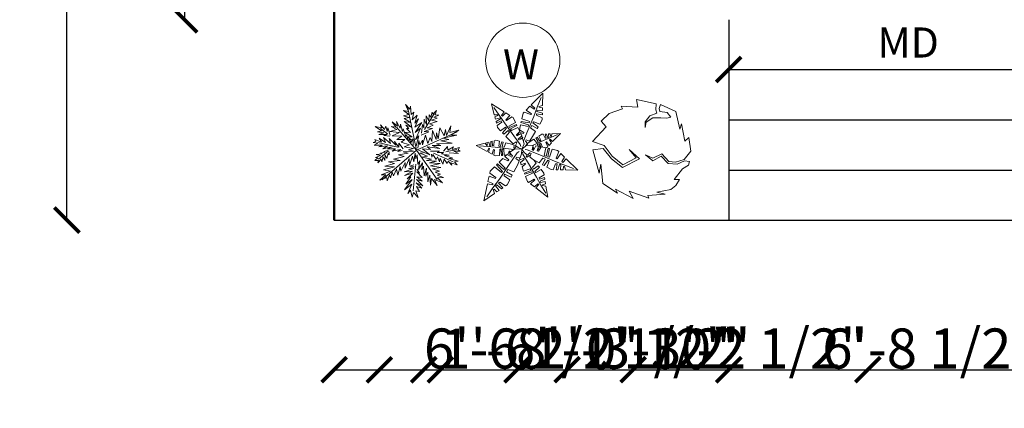
# Model space of a CAD drawing. Units: inches. Extents: x 2169 to 2662, y 1518 to 2151.
# Tile 1 of 6: x 2201 to 2398, y 1518 to 1596. Entities that reach past the tile are written whole.
import ezdxf

# ---------------------------------------------------------------- set-up
doc = ezdxf.new("R2010")
doc.units = ezdxf.units.IN
for name, color, linetype, lineweight in [('A-ANNO-DIMS', 2, 'Continuous', 18), ('A-ANNO-SYMB', 7, 'Continuous', 18), ('CAY', 94, 'Continuous', 18), ('L-PLNT-BEDS', 94, 'Continuous', 25), ('Steps', 50, 'Continuous', 25), ('Walls', 7, 'Continuous', 50)]:
    doc.layers.add(name, color=color, linetype=linetype, lineweight=lineweight)
doc.styles.add('ATT', font='romans.shx')
doc.styles.get("Standard").update_dxf_attribs({"font": 'arial.ttf'})
doc.dimstyles.get("Standard").update_dxf_attribs({"dimtxt": 8, "dimasz": 5, "dimexe": 0.18, "dimexo": 0.0625, "dimgap": 0.09, "dimtad": 1, "dimdec": 1, "dimzin": 0, "dimdsep": 46, "dimlunit": 4, "dimtxsty": 'Standard', "dimblk": 'ARCHTICK', "dimcen": 0.09, "dimse1": 1, "dimse2": 1, "dimadec": 0, "dimazin": 0, "dimtfac": 1, "dimtdec": 1, "dimtofl": 0, "dimtmove": 0, "dimatfit": 3, "dimfxl": 1, "dimtolj": 1, "dimtzin": 0, "dimarcsym": 0})

# ---------------------------------------------------------------- blocks, each defined once
blk = doc.blocks.new('_ArchTick')
at = {"color": 0, "linetype": 'ByBlock', "const_width": 0.15}
blk.add_lwpolyline([(-0.5, -0.5), (0.5, 0.5)], dxfattribs=at)
blk = doc.blocks.new('*D4')
at = {"layer": 'A-ANNO-DIMS', "color": 0, "lineweight": -2, "transparency": 16777216}
blk.add_line((2210.62, 1555.6), (2210.62, 2111.6), dxfattribs=at)
at = {"layer": 'Defpoints', "color": 0, "transparency": 16777216}
for p in [(2210.62, 2111.6), (2263.98, 2111.6), (2263.98, 1555.6)]:
    blk.add_point(p, dxfattribs=at)
at = {"layer": 'A-ANNO-DIMS', "color": 0, "lineweight": -2, "transparency": 16777216, "xscale": 5, "yscale": 5, "zscale": 5}
for p, rotation in [((2210.62, 2111.6), 90), ((2210.62, 1555.6), 270)]:
    blk.add_blockref('_ArchTick', p, dxfattribs=dict(at, rotation=rotation))
at = {"layer": 'A-ANNO-DIMS', "color": 0, "transparency": 16777216, "insert": (2206.45, 1833.6), "char_height": 8, "attachment_point": 5, "rotation": 90}
blk.add_mtext('\\A1;46\'-4"', dxfattribs=at)
blk = doc.blocks.new('A$C6FA1418A')
at = {"layer": 'CAY'}
for p, q in [((311.8, 542), (377.1, 608.2)), ((345.5, 529.3), (368, 583.5)), ((377.1, 608.2), (375.4, 538.5)), ((86.9, 547.5), (102.6, 486.1)), ((158.2, 502.2), (86.9, 547.5)), ((131, 484), (99.9, 527.4)), ((143.9, 481), (158.2, 502.2)), ((265, 494.4), (271.8, 501.4)), ((271.8, 501.4), (308.5, 486.6)), ((282.9, 512.6), (303.5, 533.5)), ((312.5, 491.8), (282.9, 512.6)), ((303.5, 533.5), (327.3, 517.9)), ((332.4, 522.8), (311.8, 542)), ((325.7, 475.6), (345.5, 529.3)), ((327.3, 517.9), (332.4, 522.8)), ((344.5, 511.9), (343.7, 504.6)), ((343.7, 504.6), (374.3, 495)), ((374.7, 510), (344.5, 511.9)), ((375.4, 538.5), (354.2, 533.2)), ((354.2, 533.2), (355.2, 527.8)), ((355.2, 527.8), (375.1, 525)), ((375.1, 525), (374.7, 510)), ((102.6, 486.1), (122.6, 485.7)), ((122.7, 480.8), (105.7, 474.2)), ((105.7, 474.2), (109.1, 461)), ((109.1, 461), (135.5, 468.9)), ((137.6, 462.5), (112.5, 447.8)), ((112.5, 447.8), (114.8, 439)), ((112.5, 447.8), (114.8, 439)), ((114.8, 439), (142.5, 451.3)), ((122.6, 485.7), (122.7, 480.8)), ((159.6, 440.6), (131, 484)), ((135.5, 468.9), (137.6, 462.5)), ((142.5, 451.3), (145.2, 444)), ((149.5, 477.7), (143.9, 481)), ((167.4, 496.4), (149.5, 477.7)), ((189.9, 482.2), (167.4, 496.4)), ((167.9, 457.6), (189.9, 482.2)), ((172.5, 453.8), (167.9, 457.6)), ((202, 474.5), (172.5, 453.8)), ((209.5, 469.7), (202, 474.5)), ((222.1, 443.1), (209.5, 469.7)), ((253.4, 441.4), (254.7, 447.5)), ((253.4, 441.4), (254.7, 447.5)), ((254.7, 447.5), (300.6, 439.7)), ((258, 462.8), (265, 494.4)), ((302.9, 447.9), (258, 462.8)), ((286.6, 384.4), (325.7, 475.6)), ((300.6, 439.7), (302.9, 447.9)), ((308.5, 486.6), (312.5, 491.8)), ((325.3, 446.7), (319.5, 439.5)), ((359.1, 432.4), (325.3, 446.7)), ((341.4, 491.4), (340.3, 482.9)), ((340.3, 482.9), (373.7, 468.8)), ((374.1, 485), (341.4, 491.4)), ((373.4, 457.4), (359.1, 432.4)), ((373.7, 468.8), (373.4, 457.4)), ((374.3, 495), (374.1, 485)), ((374.3, 495), (374.1, 485)), ((145.2, 444), (118.4, 424.7)), ((118.4, 424.7), (121, 414.7)), ((121, 414.7), (138.8, 395.4)), ((138.8, 395.4), (165.9, 415.1)), ((172.5, 409.9), (149.2, 384.2)), ((155.9, 377), (180.3, 397.8)), ((212.9, 367.8), (159.6, 440.6)), ((165.9, 415.1), (172.5, 409.9)), ((180.3, 397.8), (188.5, 387.2)), ((185.5, 420.7), (222.1, 443.1)), ((189.1, 413.9), (185.5, 420.7)), ((228.2, 430.2), (189.1, 413.9)), ((194.8, 405.7), (230.6, 425.1)), ((199.6, 397), (194.8, 405.7)), ((235.8, 414.1), (199.6, 397)), ((228, 372.3), (246.7, 391.1)), ((230.6, 425.1), (228.2, 430.2)), ((230.6, 425.1), (228.2, 430.2)), ((246.7, 391.1), (235.8, 414.1)), ((244.6, 401), (250.5, 428.3)), ((269.3, 385.4), (244.6, 401)), ((250.5, 428.3), (293.7, 419)), ((296.6, 429.5), (253.4, 441.4)), ((293.7, 419), (296.6, 429.5)), ((314.1, 424.6), (307.9, 411.3)), ((307.9, 411.3), (335.3, 390.7)), ((335.3, 390.7), (313.7, 352.9)), ((345.4, 408.3), (314.1, 424.6)), ((319.5, 439.5), (350.8, 417.8)), ((350.8, 417.8), (345.4, 408.3)), ((350.8, 417.8), (345.4, 408.3)), ((83.1, 309.8), (83.7, 334.3)), ((83.7, 334.3), (91.1, 336.2)), ((83.7, 334.3), (91.1, 336.2)), ((91.1, 336.2), (93.2, 310.9)), ((99.7, 311.9), (103, 339.4)), ((103, 339.4), (111.5, 341.6)), ((111.5, 341.6), (132.9, 336.3)), ((132.9, 336.3), (129.4, 308.4)), ((149.2, 384.2), (155.9, 377)), ((149.2, 384.2), (155.9, 377)), ((188.5, 387.2), (168.5, 363.4)), ((168.5, 363.4), (195.4, 334.4)), ((195.4, 334.4), (210.1, 322.5)), ((248.6, 318.2), (212.9, 367.8)), ((230.7, 367.4), (228, 372.3)), ((252.4, 379.2), (230.7, 367.4)), ((238.1, 371.4), (241.5, 386.8)), ((258.5, 366.3), (238.2, 348.9)), ((238.2, 348.9), (242.3, 343.6)), ((241.5, 386.8), (267.7, 379.6)), ((242.3, 343.6), (262.3, 352.7)), ((259.6, 351.5), (244.7, 354.5)), ((258.5, 366.3), (252.4, 379.2)), ((254.5, 362.9), (264.2, 357.9)), ((264.2, 357.9), (261.1, 351.2)), ((271.2, 321.1), (262.3, 352.7)), ((266.8, 336.9), (286.6, 384.4)), ((267.7, 379.6), (269.3, 385.4)), ((278.7, 337.5), (281.8, 344.2)), ((290.9, 323.7), (278.7, 337.5)), ((281.8, 344.2), (300.9, 336.5)), ((325.5, 347.7), (299.5, 331.8)), ((313.7, 352.9), (300.9, 336.5)), ((322.1, 313.5), (385, 342.5)), ((340.4, 328.9), (325.5, 347.7)), ((344.2, 359), (337.7, 355)), ((344.2, 359), (337.7, 355)), ((337.7, 355), (349.7, 333.5)), ((349.7, 333.5), (340.4, 328.9)), ((360, 337.5), (344.2, 359)), ((371.4, 375.6), (354.2, 365.1)), ((354.2, 365.1), (364.9, 341.7)), ((364.9, 341.7), (360, 337.5)), ((379.4, 376), (371.4, 375.6)), ((389.9, 352.9), (379.4, 376)), ((385, 342.5), (422.2, 357.5)), ((395.8, 353.8), (389.9, 352.9)), ((397.7, 376.9), (390.7, 376.6)), ((397.7, 376.9), (390.7, 376.6)), ((390.7, 376.6), (395.8, 353.8)), ((393.1, 330.8), (396.6, 333.7)), ((396.6, 333.7), (411.8, 313.3)), ((405, 355.7), (397.7, 376.9)), ((410.1, 356.4), (405, 355.7)), ((418.6, 378), (408.2, 377.5)), ((408.2, 377.5), (410.1, 356.4)), ((414.6, 344.5), (417.9, 348.2)), ((426, 328.1), (414.6, 344.5)), ((417.9, 348.2), (431.7, 334.2)), ((421, 364.2), (418.6, 378)), ((424.8, 363.6), (421, 364.2)), ((422.2, 357.5), (459.6, 374.2)), ((428.1, 378.5), (424.8, 363.6)), ((476.7, 381), (428.1, 378.5)), ((431.7, 334.2), (476.7, 381)), ((0, 312.5), (51.5, 325.9)), ((62.3, 278.5), (0, 312.5)), ((64.6, 306), (20, 311.1)), ((51.5, 325.9), (59.9, 311.5)), ((59.9, 311.5), (63.6, 313.4)), ((61.5, 328.5), (72.6, 331.4)), ((63.6, 313.4), (61.5, 328.5)), ((72.1, 297.7), (62.3, 278.5)), ((108.2, 302.7), (64.6, 306)), ((70.3, 274.2), (76.7, 294.9)), ((76.7, 294.9), (72.1, 297.7)), ((72.6, 331.4), (77.5, 308.9)), ((77.5, 308.9), (83.1, 309.8)), ((99, 289.6), (90, 263.5)), ((93.2, 310.9), (99.7, 311.9)), ((103.7, 287.8), (99, 289.6)), ((100.6, 257.7), (103.7, 287.8)), ((183.3, 293.2), (108.2, 302.7)), ((129.4, 308.4), (135.9, 305.7)), ((133.3, 291.8), (131.8, 255.7)), ((139.8, 291.8), (133.3, 291.8)), ((135.9, 305.7), (145.3, 333.3)), ((143.7, 256.5), (139.8, 291.8)), ((145.3, 333.3), (153.4, 331.3)), ((145.3, 333.3), (153.4, 331.3)), ((153.4, 331.3), (148, 304.9)), ((148, 304.9), (159.1, 303.2)), ((156.4, 291.1), (148.1, 291)), ((148.1, 291), (148.4, 256.8)), ((158.6, 257.4), (156.4, 291.1)), ((159.1, 303.2), (168.4, 327.6)), ((168.4, 327.6), (200.7, 319.7)), ((186.2, 280.2), (180, 258.8)), ((212.7, 289.7), (183.3, 293.2)), ((190.8, 280.3), (186.2, 280.2)), ((219.4, 294.5), (188, 272.1)), ((190.9, 274.1), (190.8, 280.3)), ((200.7, 319.7), (215.5, 313.7)), ((225.4, 333.2), (210.1, 322.5)), ((213.8, 298.1), (215.5, 313.7)), ((219.4, 297.2), (213.8, 298.1)), ((226.9, 309.1), (219.4, 297.2)), ((257.6, 291.5), (219.4, 294.5)), ((221.6, 313.2), (229.5, 327.9)), ((221.6, 313.2), (237.4, 300.4)), ((229.5, 327.9), (225.4, 333.2)), ((242.3, 278.7), (231.7, 270.7)), ((237.4, 300.4), (257.6, 291.5)), ((251.9, 307.4), (248.6, 318.2)), ((255.8, 265.5), (257.6, 291.5)), ((257.6, 291.5), (271.2, 321.1)), ((257.6, 291.5), (286, 313.4)), ((272.3, 272.1), (257.6, 291.5)), ((276.2, 289.3), (288.5, 288.5)), ((290.9, 323.7), (277.1, 306.1)), ((282.4, 312.9), (283.9, 311.7)), ((286, 313.4), (322, 311.8)), ((288.5, 288.5), (350.5, 262.6)), ((292.4, 313.1), (288.9, 321.2)), ((299.5, 331.8), (290.4, 324.3)), ((317.3, 288.1), (322, 311.8)), ((324, 285), (317.3, 288.1)), ((318.6, 311.9), (322.1, 313.5)), ((319, 300.2), (323.1, 301.4)), ((323.6, 285.2), (319, 300.2)), ((323.1, 301.4), (328.4, 293.5)), ((337.5, 311.1), (324, 285)), ((337.5, 311.1), (352.8, 307.8)), ((352.8, 307.8), (345.7, 281.6)), ((345.7, 281.6), (351.5, 280)), ((346.1, 319.1), (353.4, 321.3)), ((348.6, 308.7), (346.1, 319.1)), ((347.3, 287.6), (353.5, 289.1)), ((353.5, 289.1), (350.7, 300.1)), ((351.5, 280), (367, 304.7)), ((353.4, 321.3), (361.3, 295.5)), ((360.4, 324.4), (366.1, 326.1)), ((365, 301.4), (360.4, 324.4)), ((366.1, 326.1), (374.5, 303.1)), ((367, 304.7), (394.4, 298.8)), ((394.4, 298.8), (385.1, 255.7)), ((404.1, 305.4), (393.1, 330.8)), ((393.4, 299), (399.4, 300.5)), ((395.6, 252.8), (407.4, 296)), ((399.4, 300.5), (404.1, 305.4)), ((413.5, 294.7), (405.8, 248.8)), ((407.4, 296), (413.5, 294.7)), ((407.4, 296), (413.5, 294.7)), ((411.8, 313.3), (426, 328.1)), ((414, 246.5), (428.8, 291.3)), ((428.8, 291.3), (460.4, 284.5)), ((460.4, 284.5), (467.4, 277.7)), ((90, 263.5), (70.3, 274.2)), ((107.1, 254.1), (100.6, 257.7)), ((131.8, 255.7), (107.1, 254.1)), ((151.8, 239.4), (130.7, 218.2)), ((148.4, 256.8), (143.7, 256.5)), ((148.4, 256.8), (143.7, 256.5)), ((180.1, 226.3), (151.8, 239.4)), ((170.4, 258.2), (158.6, 257.4)), ((174.6, 262.4), (162.7, 250.5)), ((162.7, 250.5), (184.4, 231.2)), ((174.6, 262.4), (201.9, 246.9)), ((184.4, 231.2), (180.1, 226.3)), ((206.1, 253.6), (188, 272.1)), ((191.1, 259.5), (191, 269.1)), ((199.7, 260.1), (191.1, 259.5)), ((231.7, 270.7), (191.2, 211.3)), ((201.9, 246.9), (206.1, 253.6)), ((228.6, 245.7), (224.4, 239.1)), ((224.4, 239.1), (242.4, 226.4)), ((248, 242.9), (228.6, 245.7)), ((235.2, 205.4), (242.4, 226.4)), ((245.2, 243.3), (247.5, 230.9)), ((268.2, 238.1), (247.5, 230.9)), ((248, 242.9), (255.8, 265.5)), ((250, 217.1), (271.8, 232.5)), ((261.9, 275), (264.2, 264)), ((264.2, 264), (295.3, 211.4)), ((271.8, 232.5), (268.2, 238.1)), ((289.9, 258.3), (272.3, 272.1)), ((287.4, 260.3), (282.3, 252.6)), ((282.3, 252.6), (286, 247)), ((286, 247), (302.2, 256.3)), ((289.9, 258.3), (303.7, 270.5)), ((304.9, 253.7), (302.2, 256.3)), ((310.4, 267.4), (302.7, 248.3)), ((319.1, 235.5), (302.7, 248.3)), ((303.7, 270.5), (310.4, 267.4)), ((356.9, 214), (319.1, 235.5)), ((339.9, 211.8), (323.5, 233)), ((350.5, 262.6), (441.7, 223.8)), ((377.4, 241.4), (356.9, 214)), ((374.6, 204), (390.8, 235.3)), ((390.8, 235.3), (377.4, 241.4)), ((405.7, 229.9), (384, 198.6)), ((385.1, 255.7), (395.6, 252.8)), ((398.6, 190.3), (412.9, 224.2)), ((412.9, 224.2), (405.7, 229.9)), ((405.8, 248.8), (414, 246.5)), ((441.7, 223.8), (495.4, 204.1)), ((467.4, 277.7), (452.7, 240.9)), ((452.7, 240.9), (457.9, 237)), ((457.9, 237), (478.6, 266.6)), ((478.6, 266.6), (499.6, 246.1)), ((499.6, 246.1), (484, 222.3)), ((484, 222.3), (488.9, 217.2)), ((488.9, 217.2), (508, 237.8)), ((508, 237.8), (574.3, 172.7)), ((79.9, 166.7), (77.6, 156.6)), ((104.2, 191.4), (79.9, 166.7)), ((143.7, 159.8), (104.2, 191.4)), ((120.7, 208), (116, 203.3)), ((120.7, 208), (116, 203.3)), ((116, 203.3), (149.7, 166.6)), ((156.5, 176.2), (120.7, 208)), ((130.7, 218.2), (164.2, 184.9)), ((191.2, 211.3), (132.1, 123.3)), ((164.2, 184.9), (156.5, 176.2)), ((171.1, 163.3), (179.5, 176.6)), ((179.5, 176.6), (213.8, 164)), ((213.8, 164), (235.2, 205.4)), ((250, 217.1), (254.9, 203.7)), ((254.9, 203.7), (277.6, 213.4)), ((279.8, 208.4), (259.5, 191.3)), ((259.5, 191.3), (268.3, 167.4)), ((268.3, 167.4), (305.9, 181.2)), ((309.8, 172.1), (272.5, 156)), ((277.6, 213.4), (279.8, 208.4)), ((295.3, 211.4), (341.7, 134.3)), ((305.9, 181.2), (309.8, 172.1)), ((317.8, 189.9), (339.9, 211.8)), ((325, 178.6), (317.8, 189.9)), ((351.1, 197.2), (325, 178.6)), ((331.7, 165.9), (357.2, 189.4)), ((366.5, 177.3), (337.8, 160.2)), ((357.2, 189.4), (351.1, 197.2)), ((357.2, 189.4), (351.1, 197.2)), ((382.4, 156.6), (366.5, 177.3)), ((384, 198.6), (374.6, 204)), ((384, 198.6), (374.6, 204)), ((423.6, 176.1), (398.6, 190.3)), ((435, 175.8), (423.6, 176.1)), ((449, 209.2), (435, 175.8)), ((457.5, 208.2), (449, 209.2)), ((451.2, 175.5), (457.5, 208.2)), ((461.2, 175.2), (451.2, 175.5)), ((461.2, 175.2), (451.2, 175.5)), ((470.7, 205.8), (461.2, 175.2)), ((478, 205.1), (470.7, 205.8)), ((476.2, 174.9), (478, 205.1)), ((491.2, 174.6), (476.2, 174.9)), ((494, 194.4), (491.2, 174.6)), ((499.3, 195.5), (494, 194.4)), ((495.4, 204.1), (549.6, 181.7)), ((504.7, 174.3), (499.3, 195.5)), ((574.3, 172.7), (504.7, 174.3)), ((74, 140.1), (67.2, 109.4)), ((109.9, 125.6), (74, 140.1)), ((77.6, 156.6), (112.3, 132.2)), ((132.1, 123.3), (95.5, 74.2)), ((112.3, 132.2), (109.9, 125.6)), ((149.7, 166.6), (143.7, 159.8)), ((157.7, 140.4), (160.8, 149.8)), ((190.3, 118.4), (157.7, 140.4)), ((160.8, 149.8), (198.6, 134.4)), ((203.9, 144.7), (171.1, 163.3)), ((176.2, 91), (190.3, 118.4)), ((198.6, 134.4), (203.9, 144.7)), ((198.6, 134.4), (203.9, 144.7)), ((272.5, 156), (274.4, 150.7)), ((272.5, 156), (274.4, 150.7)), ((274.4, 150.7), (314.8, 163.4)), ((317.8, 156.3), (279.3, 137.4)), ((279.3, 137.4), (289.5, 109.7)), ((296.5, 104.4), (327.7, 122.2)), ((331.9, 118), (307.8, 95.6)), ((314.8, 163.4), (317.8, 156.3)), ((327.7, 122.2), (331.9, 118)), ((337.8, 160.2), (331.7, 165.9)), ((341.7, 134.3), (366.3, 88.4)), ((355.8, 129.5), (384.1, 146.3)), ((357.8, 122), (355.8, 129.5)), ((386.5, 131.8), (357.8, 122)), ((361.6, 110.4), (387.9, 122.8)), ((384.1, 146.3), (382.4, 156.6)), ((387.9, 122.8), (386.5, 131.8)), ((387.9, 122.8), (386.5, 131.8)), ((64.5, 97), (43.1, 0)), ((95.5, 74.2), (60, 22.5)), ((93.7, 89.7), (64.5, 97)), ((67.2, 109.4), (95.1, 97.2)), ((95.1, 97.2), (93.7, 89.7)), ((97, 64.2), (102.4, 66.4)), ((104.6, 42), (97, 64.2)), ((102.4, 66.4), (116.5, 50.2)), ((110.5, 85.2), (116.6, 90.2)), ((129.8, 59.3), (110.5, 85.2)), ((116.5, 50.2), (129.8, 59.3)), ((116.6, 90.2), (143, 68.3)), ((127.1, 100), (134.1, 105.9)), ((151.9, 74.4), (127.1, 100)), ((134.1, 105.9), (166.1, 84.1)), ((143, 68.3), (151.9, 74.4)), ((143, 68.3), (151.9, 74.4)), ((166.1, 84.1), (176.2, 91)), ((289.5, 109.7), (296.5, 104.4)), ((307.8, 95.6), (329, 79.4)), ((329, 79.4), (348.4, 96.4)), ((353.7, 92.6), (337.5, 72.8)), ((337.5, 72.8), (404.5, 21.4)), ((348.4, 96.4), (353.7, 92.6)), ((363.2, 103.9), (361.6, 110.4)), ((390.1, 109.4), (363.2, 103.9)), ((366.3, 88.4), (393.3, 42.5)), ((374.5, 86), (374.8, 90.9)), ((394.3, 83.8), (374.5, 86)), ((374.8, 90.9), (392.3, 95.9)), ((392.3, 95.9), (390.1, 109.4)), ((404.5, 21.4), (394.3, 83.8)), ((43.1, 0), (104.6, 42))]:
    blk.add_line(p, q, dxfattribs=at)
blk = doc.blocks.new('12PPLT15')
at = {"color": 0, "linetype": 'ByBlock'}
for p, q in [((0.013, -0.001), (-0.088, 0.491)), ((0.105, 0.233), (0.218, 0.416)), ((-0.311, 0.181), (-0.394, 0.245)), ((0.013, -0.001), (-0.211, 0.261)), ((0.013, -0.001), (0.471, 0.206)), ((-0.197, 0.032), (-0.424, 0.087)), ((0.344, -0.02), (0.467, 0.009)), ((-0.304, -0.006), (-0.415, -0.1)), ((0.013, -0.001), (-0.373, -0.336)), ((0.013, -0.001), (0.245, -0.333)), ((0.205, -0.033), (0.429, -0.132)), ((0.006, -0.159), (-0.023, -0.458))]:
    blk.add_line(p, q, dxfattribs=at)
for points in [[(0.008, 0.049), (0.041, 0.162), (0.002, 0.122), (0.057, 0.248), (-0.001, 0.2), (0.073, 0.313), (-0.007, 0.258), (0.035, 0.352), (-0.007, 0.306), (0.021, 0.394), (-0.034, 0.342), (-0.015, 0.43), (-0.046, 0.403), (-0.053, 0.497), (-0.063, 0.461), (-0.111, 0.516), (-0.076, 0.436), (-0.134, 0.449), (-0.072, 0.403), (-0.134, 0.388), (-0.069, 0.367), (-0.126, 0.359), (-0.053, 0.313), (-0.126, 0.323), (-0.042, 0.261), (-0.105, 0.281), (-0.072, 0.245), (-0.101, 0.245), (-0.053, 0.2), (-0.12, 0.204), (-0.034, 0.149), (-0.092, 0.151), (-0.04, 0.113)], [(0.069, 0.191), (0.083, 0.29), (0.096, 0.252), (0.099, 0.348), (0.125, 0.29), (0.121, 0.388), (0.154, 0.332), (0.157, 0.397), (0.176, 0.374), (0.19, 0.43), (0.199, 0.407), (0.238, 0.449), (0.224, 0.397), (0.266, 0.394), (0.209, 0.374), (0.247, 0.361), (0.182, 0.338), (0.245, 0.323), (0.161, 0.296), (0.203, 0.281), (0.134, 0.252), (0.193, 0.245), (0.102, 0.212), (0.154, 0.206), (0.067, 0.168)], [(-0.289, 0.158), (-0.356, 0.164), (-0.323, 0.177), (-0.411, 0.177), (-0.356, 0.197), (-0.427, 0.206), (-0.382, 0.219), (-0.453, 0.268), (-0.379, 0.252), (-0.394, 0.284), (-0.346, 0.233), (-0.331, 0.271), (-0.317, 0.212), (-0.311, 0.252), (-0.285, 0.17)], [(-0.023, 0.057), (-0.023, 0.126), (-0.05, 0.087), (-0.065, 0.126), (-0.076, 0.103), (-0.098, 0.174), (-0.107, 0.155), (-0.136, 0.239), (-0.143, 0.21), (-0.166, 0.294), (-0.17, 0.248), (-0.214, 0.323), (-0.201, 0.271), (-0.262, 0.319), (-0.22, 0.258), (-0.272, 0.268), (-0.208, 0.233), (-0.289, 0.212), (-0.178, 0.2), (-0.26, 0.162), (-0.153, 0.158), (-0.208, 0.12), (-0.117, 0.12), (-0.159, 0.09), (-0.065, 0.061), (-0.126, 0.038), (-0.021, 0.019), (-0.078, 0.003), (-0.021, -0.012), (-0.136, -0.02), (-0.082, -0.035), (-0.191, -0.054), (-0.126, -0.071), (-0.247, -0.1), (-0.17, -0.117), (-0.304, -0.132), (-0.233, -0.152), (-0.344, -0.181), (-0.233, -0.19), (-0.359, -0.223), (-0.279, -0.236), (-0.385, -0.278), (-0.331, -0.278), (-0.401, -0.339), (-0.321, -0.31), (-0.317, -0.345), (-0.291, -0.278), (-0.281, -0.314), (-0.262, -0.249), (-0.247, -0.291), (-0.214, -0.213), (-0.197, -0.284), (-0.17, -0.184), (-0.162, -0.239), (-0.114, -0.139), (-0.114, -0.203), (-0.069, -0.094), (-0.065, -0.171), (-0.03, -0.068), (-0.015, -0.132), (-0.001, -0.035), (0.006, -0.098), (0.021, -0.052), (0.027, -0.159), (0.05, -0.119), (0.038, -0.217), (0.083, -0.142), (0.073, -0.223), (0.092, -0.181), (0.099, -0.291), (0.125, -0.203), (0.119, -0.294), (0.14, -0.249), (0.14, -0.358), (0.163, -0.281), (0.17, -0.397), (0.182, -0.32), (0.245, -0.4), (0.215, -0.333), (0.306, -0.368), (0.251, -0.314), (0.318, -0.31), (0.247, -0.284), (0.283, -0.272), (0.224, -0.249), (0.274, -0.236), (0.193, -0.209), (0.287, -0.194), (0.17, -0.178), (0.28, -0.152), (0.161, -0.142), (0.241, -0.123), (0.125, -0.117), (0.182, -0.1), (0.079, -0.081), (0.138, -0.068), (0.05, -0.033), (0.09, -0.029)], [(0.038, 0), (0.163, -0.052), (0.083, 0.015), (0.17, 0.007), (0.134, 0.036), (0.276, 0.019), (0.19, 0.051), (0.289, 0.051), (0.238, 0.071), (0.415, 0.08), (0.289, 0.107), (0.379, 0.12), (0.309, 0.135), (0.467, 0.168), (0.396, 0.17), (0.49, 0.226), (0.389, 0.2), (0.4, 0.275), (0.354, 0.164), (0.341, 0.233), (0.325, 0.162), (0.276, 0.252), (0.257, 0.126), (0.238, 0.197), (0.234, 0.12), (0.193, 0.223), (0.186, 0.099), (0.167, 0.141), (0.14, 0.074), (0.115, 0.17), (0.083, 0.061), (0.083, 0.113), (0.05, 0.061), (0.041, 0.11), (0.027, 0.022)], [(-0.136, 0.015), (-0.185, 0.078), (-0.185, 0.032), (-0.233, 0.099), (-0.22, 0.055), (-0.295, 0.132), (-0.279, 0.074), (-0.359, 0.141), (-0.337, 0.087), (-0.408, 0.135), (-0.382, 0.09), (-0.457, 0.122), (-0.446, 0.097), (-0.476, 0.087), (-0.424, 0.078), (-0.466, 0.055), (-0.369, 0.055), (-0.411, 0.038), (-0.314, 0.049), (-0.366, 0.015), (-0.26, 0.036), (-0.314, 0.013), (-0.224, 0.015), (-0.26, -0.012), (-0.166, 0.009), (-0.197, -0.016), (-0.149, -0.004)], [(0.318, -0.01), (0.364, 0.042), (0.367, 0), (0.431, 0.036), (0.415, 0.009), (0.499, 0.029), (0.483, 0.003), (0.506, -0.01), (0.435, -0.01), (0.486, -0.039), (0.383, -0.029)], [(-0.311, -0.004), (-0.356, -0.016), (-0.34, -0.023), (-0.394, -0.033), (-0.373, -0.042), (-0.44, -0.048), (-0.394, -0.062), (-0.45, -0.084), (-0.421, -0.087), (-0.457, -0.117), (-0.415, -0.117), (-0.424, -0.142), (-0.385, -0.1), (-0.379, -0.132), (-0.363, -0.075), (-0.344, -0.117), (-0.34, -0.054), (-0.321, -0.094), (-0.308, -0.035), (-0.295, -0.054), (-0.295, -0.02)], [(0.17, -0.012), (0.274, -0.012), (0.245, -0.026), (0.318, -0.026), (0.295, -0.042), (0.383, -0.058), (0.328, -0.062), (0.425, -0.09), (0.377, -0.094), (0.483, -0.126), (0.442, -0.132), (0.471, -0.165), (0.4, -0.142), (0.412, -0.171), (0.37, -0.123), (0.36, -0.152), (0.325, -0.1), (0.312, -0.159), (0.28, -0.09), (0.274, -0.132), (0.251, -0.075), (0.234, -0.106), (0.199, -0.048), (0.186, -0.081), (0.182, -0.045)], [(-0.017, -0.165), (-0.063, -0.181), (-0.011, -0.188), (-0.078, -0.209), (-0.015, -0.207), (-0.124, -0.245), (-0.03, -0.236), (-0.12, -0.287), (-0.027, -0.261), (-0.092, -0.322), (-0.05, -0.303), (-0.107, -0.385), (-0.034, -0.333), (-0.12, -0.448), (-0.04, -0.385), (-0.084, -0.49), (-0.053, -0.452), (-0.034, -0.53), (-0.021, -0.477), (0.031, -0.533), (0.006, -0.458), (0.048, -0.465), (0.012, -0.41), (0.073, -0.429), (0.008, -0.368), (0.086, -0.404), (0.012, -0.333), (0.079, -0.349), (0.019, -0.303), (0.079, -0.307), (0.019, -0.245), (0.048, -0.259), (0.019, -0.213)]]:
    blk.add_lwpolyline(points, dxfattribs=at)
at = {"color": 0, "linetype": 'ByBlock', "style": 'ATT'}
for tag, p, flags in [('ITEM', (-1, -3.75), 3), ('ROOM_NUMBER', (-1, -5.083), 1)]:
    blk.add_attdef(tag, p, '', height=1, dxfattribs=dict(at, flags=flags))
blk = doc.blocks.new('Archi.Space.tree546513')
for p, q in [((327.581, 76.31, 0), (327.646, 75.982, 0)), ((328.421, 76.123, 0), (327.581, 76.31, 0)), ((326.995, 75.904, 0), (326.428, 75.717, 0)), ((326.943, 76.029, 0), (326.995, 75.904, 0)), ((327.646, 75.982, 0), (326.943, 76.029, 0)), ((328.408, 75.873, 0), (328.421, 76.123, 0)), ((328.447, 75.733, 0), (328.408, 75.873, 0)), ((328.603, 76.092, 0), (328.551, 75.92, 0)), ((328.551, 75.92, 0), (328.577, 75.795, 0)), ((329.254, 75.795, 0), (328.603, 76.092, 0)), ((326.428, 75.717, 0), (326.09, 75.389, 0)), ((327.958, 75.358, 0), (328.148, 75.608, 0)), ((328.278, 75.53, 0), (327.997, 75.343, 0)), ((328.148, 75.608, 0), (328.447, 75.733, 0)), ((328.616, 75.53, 0), (328.278, 75.53, 0)), ((328.577, 75.795, 0), (328.889, 75.748, 0)), ((328.863, 75.514, 0), (328.616, 75.53, 0)), ((329.032, 75.561, 0), (328.863, 75.514, 0)), ((328.889, 75.748, 0), (329.032, 75.561, 0)), ((329.423, 75.046, 0), (329.254, 75.795, 0)), ((326.298, 75.155, 0), (325.726, 74.521, 0)), ((326.09, 75.389, 0), (326.298, 75.155, 0)), ((327.958, 75.124, 0), (327.958, 75.358, 0)), ((327.997, 75.343, 0), (327.958, 75.124, 0)), ((329.488, 75.28, 0), (329.423, 75.046, 0)), ((329.488, 75.28, 0), (329.488, 75.28, 0)), ((329.626, 74.536, 0), (329.488, 75.28, 0)), ((329.795, 74.692, 0), (329.626, 74.536, 0)), ((329.886, 74.115, 0), (329.795, 74.692, 0)), ((325.726, 74.521, 0), (326.22, 74.365, 0)), ((326.168, 74.224, 0), (325.739, 74.178, 0)), ((326.532, 73.787, 0), (326.168, 74.224, 0)), ((326.22, 74.365, 0), (326.558, 73.912, 0)), ((327.268, 74.193, 0), (327.711, 73.787, 0)), ((327.568, 73.834, 0), (327.268, 74.193, 0)), ((325.739, 74.178, 0), (325.999, 73.184, 0)), ((326.995, 73.429, 0), (326.532, 73.787, 0)), ((326.558, 73.912, 0), (327.008, 73.538, 0)), ((327.711, 73.787, 0), (326.995, 73.429, 0)), ((327.008, 73.538, 0), (327.568, 73.834, 0)), ((327.971, 73.959, 0), (328.278, 73.819, 0)), ((328.278, 73.709, 0), (327.971, 73.959, 0)), ((328.278, 73.819, 0), (328.655, 74.006, 0)), ((328.629, 73.912, 0), (328.278, 73.709, 0)), ((328.928, 73.6, 0), (328.629, 73.912, 0)), ((328.655, 74.006, 0), (328.954, 73.678, 0)), ((329.24, 73.647, 0), (329.605, 73.772, 0)), ((329.605, 73.772, 0), (329.886, 74.115, 0)), ((325.999, 73.184, 0), (326.077, 73.569, 0)), ((326.077, 73.569, 0), (326.155, 72.747, 0)), ((329.306, 73.569, 0), (328.928, 73.6, 0)), ((328.954, 73.678, 0), (329.24, 73.647, 0)), ((329.175, 72.919, 0), (329.527, 73.366, 0)), ((329.613, 73.709, 0), (329.306, 73.569, 0)), ((329.527, 73.366, 0), (329.782, 73.522, 0)), ((329.834, 73.678, 0), (329.613, 73.709, 0)), ((329.782, 73.522, 0), (329.834, 73.678, 0)), ((326.155, 72.747, 0), (326.774, 72.342, 0)), ((329.045, 72.498, 0), (329.254, 72.669, 0)), ((329.41, 72.919, 0), (329.175, 72.919, 0)), ((329.254, 72.669, 0), (329.41, 72.919, 0)), ((326.696, 72.513, 0), (327.438, 72.108, 0)), ((326.774, 72.342, 0), (326.696, 72.513, 0)), ((327.281, 72.42, 0), (328.114, 72.123, 0)), ((327.438, 72.108, 0), (327.281, 72.42, 0)), ((328.062, 72.248, 0), (328.798, 72.295, 0)), ((328.114, 72.123, 0), (328.062, 72.248, 0)), ((328.447, 72.388, 0), (329.045, 72.498, 0)), ((328.798, 72.295, 0), (328.447, 72.388, 0))]:
    blk.add_line(p, q)
blk = doc.blocks.new('*D41')
at = {"layer": 'A-ANNO-DIMS', "color": 0, "lineweight": -2, "transparency": 16777216}
for p, q in [((2342.72, 1585.67), (2408.92, 1585.67)), ((2408.92, 1585.67), (2502.68, 1585.67))]:
    blk.add_line(p, q, dxfattribs=at)
at = {"layer": 'Defpoints', "color": 0, "transparency": 16777216}
for p in [(2342.72, 1595.6), (2408.92, 1595.6), (2408.92, 1585.67)]:
    blk.add_point(p, dxfattribs=at)
at = {"layer": 'A-ANNO-DIMS', "color": 0, "lineweight": -2, "transparency": 16777216, "xscale": 5, "yscale": 5, "zscale": 5, "rotation": 180}
blk.add_blockref('_ArchTick', (2342.72, 1585.67), dxfattribs=at)
at = {"layer": 'A-ANNO-DIMS', "color": 0, "lineweight": -2, "transparency": 16777216, "xscale": 5, "yscale": 5, "zscale": 5}
blk.add_blockref('_ArchTick', (2408.92, 1585.67), dxfattribs=at)
at = {"layer": 'A-ANNO-DIMS', "color": 0, "transparency": 16777216, "insert": (2458.3, 1589.9), "char_height": 8, "attachment_point": 5}
blk.add_mtext('\\A1;MAIN DOOR 5\'-6"', dxfattribs=at)
blk = doc.blocks.new('*D56')
at = {"layer": 'A-ANNO-DIMS', "color": 0, "lineweight": -2, "transparency": 16777216}
blk.add_line((2342.72, 1525.75), (2422.98, 1525.75), dxfattribs=at)
at = {"layer": 'Defpoints', "color": 0, "transparency": 16777216}
for p in [(2342.72, 1555.6), (2422.98, 1555.6), (2422.98, 1525.75)]:
    blk.add_point(p, dxfattribs=at)
at = {"layer": 'A-ANNO-DIMS', "color": 0, "lineweight": -2, "transparency": 16777216, "xscale": 5, "yscale": 5, "zscale": 5, "rotation": 180}
blk.add_blockref('_ArchTick', (2342.72, 1525.75), dxfattribs=at)
at = {"layer": 'A-ANNO-DIMS', "color": 0, "lineweight": -2, "transparency": 16777216, "xscale": 5, "yscale": 5, "zscale": 5}
blk.add_blockref('_ArchTick', (2422.98, 1525.75), dxfattribs=at)
at = {"layer": 'A-ANNO-DIMS', "color": 0, "transparency": 16777216, "insert": (2382.85, 1529.98), "char_height": 8, "attachment_point": 5}
blk.add_mtext('\\A1;6\'-8 1/2"', dxfattribs=at)
blk = doc.blocks.new('*D57')
at = {"layer": 'A-ANNO-DIMS', "color": 0, "lineweight": -2, "transparency": 16777216}
blk.add_line((2263.98, 1525.75), (2342.72, 1525.75), dxfattribs=at)
at = {"layer": 'Defpoints', "color": 0, "transparency": 16777216}
for p in [(2263.98, 1555.6), (2342.72, 1555.6), (2342.72, 1525.75)]:
    blk.add_point(p, dxfattribs=at)
at = {"layer": 'A-ANNO-DIMS', "color": 0, "lineweight": -2, "transparency": 16777216, "xscale": 5, "yscale": 5, "zscale": 5, "rotation": 180}
blk.add_blockref('_ArchTick', (2263.98, 1525.75), dxfattribs=at)
at = {"layer": 'A-ANNO-DIMS', "color": 0, "lineweight": -2, "transparency": 16777216, "xscale": 5, "yscale": 5, "zscale": 5}
blk.add_blockref('_ArchTick', (2342.72, 1525.75), dxfattribs=at)
at = {"layer": 'A-ANNO-DIMS', "color": 0, "transparency": 16777216, "insert": (2303.35, 1529.98), "char_height": 8, "attachment_point": 5}
blk.add_mtext('\\A1;6\'-6 1/2"', dxfattribs=at)
blk = doc.blocks.new('*D58')
at = {"layer": 'A-ANNO-DIMS', "color": 0, "lineweight": -2, "transparency": 16777216}
blk.add_line((2234.13, 1595.6), (2234.13, 1646.49), dxfattribs=at)
at = {"layer": 'Defpoints', "color": 0, "transparency": 16777216}
for p in [(2234.13, 1646.49), (2263.98, 1646.49), (2263.98, 1595.6)]:
    blk.add_point(p, dxfattribs=at)
at = {"layer": 'A-ANNO-DIMS', "color": 0, "lineweight": -2, "transparency": 16777216, "xscale": 5, "yscale": 5, "zscale": 5}
for p, rotation in [((2234.13, 1646.49), 90), ((2234.13, 1595.6), 270)]:
    blk.add_blockref('_ArchTick', p, dxfattribs=dict(at, rotation=rotation))
at = {"layer": 'A-ANNO-DIMS', "color": 0, "transparency": 16777216, "insert": (2229.95, 1621.05), "char_height": 8, "attachment_point": 5, "rotation": 90}
blk.add_mtext('\\A1;4\'-3"', dxfattribs=at)
blk = doc.blocks.new('*D65')
at = {"layer": 'A-ANNO-DIMS', "color": 0, "lineweight": -2, "transparency": 16777216}
for p, q in [((2263.98, 1525.75), (2281.85, 1525.75)), ((2281.85, 1525.75), (2307.54, 1525.75))]:
    blk.add_line(p, q, dxfattribs=at)
at = {"layer": 'Defpoints', "color": 0, "transparency": 16777216}
for p in [(2263.98, 1595.6), (2281.85, 1595.6), (2281.85, 1525.75)]:
    blk.add_point(p, dxfattribs=at)
at = {"layer": 'A-ANNO-DIMS', "color": 0, "lineweight": -2, "transparency": 16777216, "xscale": 5, "yscale": 5, "zscale": 5, "rotation": 180}
blk.add_blockref('_ArchTick', (2263.98, 1525.75), dxfattribs=at)
at = {"layer": 'A-ANNO-DIMS', "color": 0, "lineweight": -2, "transparency": 16777216, "xscale": 5, "yscale": 5, "zscale": 5}
blk.add_blockref('_ArchTick', (2281.85, 1525.75), dxfattribs=at)
at = {"layer": 'A-ANNO-DIMS', "color": 0, "transparency": 16777216, "insert": (2297.19, 1529.93), "char_height": 8, "attachment_point": 5}
blk.add_mtext('\\A1;1\'-6"', dxfattribs=at)
blk = doc.blocks.new('*D70')
at = {"layer": 'A-ANNO-DIMS', "color": 0, "lineweight": -2, "transparency": 16777216}
blk.add_line((2272.98, 1525.75), (2370.48, 1525.75), dxfattribs=at)
at = {"layer": 'Defpoints', "color": 0, "transparency": 16777216}
for p in [(2272.98, 1886.6), (2370.48, 1886.6), (2370.48, 1525.75)]:
    blk.add_point(p, dxfattribs=at)
at = {"layer": 'A-ANNO-DIMS', "color": 0, "lineweight": -2, "transparency": 16777216, "xscale": 5, "yscale": 5, "zscale": 5, "rotation": 180}
blk.add_blockref('_ArchTick', (2272.98, 1525.75), dxfattribs=at)
at = {"layer": 'A-ANNO-DIMS', "color": 0, "lineweight": -2, "transparency": 16777216, "xscale": 5, "yscale": 5, "zscale": 5}
blk.add_blockref('_ArchTick', (2370.48, 1525.75), dxfattribs=at)
at = {"layer": 'A-ANNO-DIMS', "color": 0, "transparency": 16777216, "insert": (2321.73, 1529.98), "char_height": 8, "attachment_point": 5}
blk.add_mtext('\\A1;8\'-1 1/2"', dxfattribs=at)
blk = doc.blocks.new('*D71')
at = {"layer": 'A-ANNO-DIMS', "color": 0, "lineweight": -2, "transparency": 16777216}
for p, q in [((2300.48, 1525.75), (2310.48, 1525.75)), ((2310.48, 1525.75), (2343.14, 1525.75))]:
    blk.add_line(p, q, dxfattribs=at)
at = {"layer": 'Defpoints', "color": 0, "transparency": 16777216}
for p in [(2300.48, 1886.6), (2310.48, 1886.6), (2310.48, 1525.75)]:
    blk.add_point(p, dxfattribs=at)
at = {"layer": 'A-ANNO-DIMS', "color": 0, "lineweight": -2, "transparency": 16777216, "xscale": 5, "yscale": 5, "zscale": 5, "rotation": 180}
blk.add_blockref('_ArchTick', (2300.48, 1525.75), dxfattribs=at)
at = {"layer": 'A-ANNO-DIMS', "color": 0, "lineweight": -2, "transparency": 16777216, "xscale": 5, "yscale": 5, "zscale": 5}
blk.add_blockref('_ArchTick', (2310.48, 1525.75), dxfattribs=at)
at = {"layer": 'A-ANNO-DIMS', "color": 0, "transparency": 16777216, "insert": (2329.31, 1529.93), "char_height": 8, "attachment_point": 5}
blk.add_mtext('\\A1;0\'-10"', dxfattribs=at)
blk = doc.blocks.new('*D74')
at = {"layer": 'A-ANNO-DIMS', "color": 0, "lineweight": -2, "transparency": 16777216}
for p, q in [((2272.98, 1525.75), (2300.48, 1525.75)), ((2300.48, 1525.75), (2345.7, 1525.75))]:
    blk.add_line(p, q, dxfattribs=at)
at = {"layer": 'Defpoints', "color": 0, "transparency": 16777216}
for p in [(2272.98, 1886.6), (2300.48, 1886.6), (2300.48, 1525.75)]:
    blk.add_point(p, dxfattribs=at)
at = {"layer": 'A-ANNO-DIMS', "color": 0, "lineweight": -2, "transparency": 16777216, "xscale": 5, "yscale": 5, "zscale": 5, "rotation": 180}
blk.add_blockref('_ArchTick', (2272.98, 1525.75), dxfattribs=at)
at = {"layer": 'A-ANNO-DIMS', "color": 0, "lineweight": -2, "transparency": 16777216, "xscale": 5, "yscale": 5, "zscale": 5}
blk.add_blockref('_ArchTick', (2300.48, 1525.75), dxfattribs=at)
at = {"layer": 'A-ANNO-DIMS', "color": 0, "transparency": 16777216, "insert": (2325.59, 1529.98), "char_height": 8, "attachment_point": 5}
blk.add_mtext('\\A1;2\'-3 1/2"', dxfattribs=at)
blk = doc.blocks.new('*D80')
at = {"layer": 'A-ANNO-DIMS', "color": 0, "lineweight": -2, "transparency": 16777216}
for p, q in [((2285.18, 1525.75), (2323.65, 1525.75)), ((2323.65, 1525.75), (2368.73, 1525.75))]:
    blk.add_line(p, q, dxfattribs=at)
at = {"layer": 'Defpoints', "color": 0, "transparency": 16777216}
for p in [(2285.18, 1638.55), (2323.65, 1638.55), (2323.65, 1525.75)]:
    blk.add_point(p, dxfattribs=at)
at = {"layer": 'A-ANNO-DIMS', "color": 0, "lineweight": -2, "transparency": 16777216, "xscale": 5, "yscale": 5, "zscale": 5, "rotation": 180}
blk.add_blockref('_ArchTick', (2285.18, 1525.75), dxfattribs=at)
at = {"layer": 'A-ANNO-DIMS', "color": 0, "lineweight": -2, "transparency": 16777216, "xscale": 5, "yscale": 5, "zscale": 5}
blk.add_blockref('_ArchTick', (2323.65, 1525.75), dxfattribs=at)
at = {"layer": 'A-ANNO-DIMS', "color": 0, "transparency": 16777216, "insert": (2348.69, 1529.98), "char_height": 8, "attachment_point": 5}
blk.add_mtext('\\A1;3\'-2 1/2"', dxfattribs=at)

msp = doc.modelspace()

# ---------------------------------------------------------------- linework, layer by layer
at = {"layer": 'A-ANNO-SYMB'}
msp.add_circle((2301.62, 1587.52), 7.42, dxfattribs=at)
at = {"layer": 'L-PLNT-BEDS'}
for p in [(2342.72, 1595.6), (2263.98, 1555.6)]:
    msp.add_line(p, (2342.72, 1555.6), dxfattribs=at)
at = {"layer": 'Steps'}
for p, q in [((2342.72, 1575.6), (2422.98, 1575.6)), ((2342.72, 1565.6), (2422.98, 1565.6)), ((2342.72, 1555.6), (2422.98, 1555.6))]:
    msp.add_line(p, q, dxfattribs=at)
at = {"layer": 'Walls'}
msp.add_line((2263.98, 2111.6), (2263.98, 1555.6), dxfattribs=at)

# ---------------------------------------------------------------- block references
at = {"layer": 'CAY'}
for name, p, xscale, yscale, zscale in [('A$C6FA1418A', (2292.29, 1559.45), 0.0353665555892609, 0.0353665555892609, 0.0353665555892609), ('12PPLT15', (2280.16, 1569.57), 17.68327779463044, 17.68327779463044, 17.68327779463044), ('Archi.Space.tree546513', (779.57, 1219.86, 0), 4.715540745234783, 4.715540745234783, 4.715540745234783)]:
    msp.add_blockref(name, p, dxfattribs=dict(at, xscale=xscale, yscale=yscale, zscale=zscale))

# ---------------------------------------------------------------- texts
at = {"layer": 'A-ANNO-SYMB'}
for s, p in [('MD', (2372.39, 1588.05)), ('W', (2297.66, 1583.72))]:
    msp.add_text(s, height=6, dxfattribs=at).set_placement(p)

# ---------------------------------------------------------------- dimensions: what is measured, and where the dimension line sits
at = {"layer": 'A-ANNO-DIMS'}
for base, p1, p2, override, picture, middle in [((2210.62, 2111.6), (2263.98, 1555.6), (2263.98, 2111.6), {"dimclrd": 0, "dimclre": 0, "dimclrt": 0}, '*D4', (2206.45, 1833.6)), ((2234.13, 1646.49), (2263.98, 1595.6), (2263.98, 1646.49), {"dimdec": 1, "dimlfac": 1, "dimrnd": 0, "dimzin": 1, "dimdsep": 46, "dimlunit": 4, "dimfrac": 2}, '*D58', (2229.95, 1621.05))]:
    dim = msp.add_linear_dim(base=base, p1=p1, p2=p2, angle=90, dimstyle='Standard', override=override, dxfattribs=at)
    dim.commit()
    dim.dimension.update_dxf_attribs({"geometry": picture, "text_midpoint": middle})
for base, p1, p2, picture, middle in [((2370.48, 1525.75), (2272.98, 1886.6), (2370.48, 1886.6), '*D70', (2321.73, 1529.98)), ((2300.48, 1525.75), (2272.98, 1886.6), (2300.48, 1886.6), '*D74', (2325.59, 1529.98)), ((2310.48, 1525.75), (2300.48, 1886.6), (2310.48, 1886.6), '*D71', (2329.31, 1529.93)), ((2323.65, 1525.75), (2285.18, 1638.55), (2323.65, 1638.55), '*D80', (2348.69, 1529.98)), ((2281.85, 1525.75), (2263.98, 1595.6), (2281.85, 1595.6), '*D65', (2297.19, 1529.93)), ((2342.72, 1525.75), (2263.98, 1555.6), (2342.72, 1555.6), '*D57', (2303.35, 1529.98)), ((2422.98, 1525.75), (2342.72, 1555.6), (2422.98, 1555.6), '*D56', (2382.85, 1529.98))]:
    dim = msp.add_linear_dim(base=base, p1=p1, p2=p2, dimstyle='Standard', override={"dimdec": 1, "dimlfac": 1, "dimrnd": 0, "dimzin": 1, "dimdsep": 46, "dimlunit": 4, "dimfrac": 2}, dxfattribs=at)
    dim.commit()
    dim.dimension.update_dxf_attribs({"geometry": picture, "text_midpoint": middle})
dim = msp.add_linear_dim(base=(2408.92, 1585.67), p1=(2342.72, 1595.6), p2=(2408.92, 1595.6), text='MAIN DOOR <>', dimstyle='Standard', override={"dimdec": 1, "dimlfac": 1, "dimrnd": 0, "dimzin": 1, "dimdsep": 46, "dimlunit": 4, "dimfrac": 2}, dxfattribs=at)
dim.commit()
dim.dimension.update_dxf_attribs({"geometry": '*D41', "text_midpoint": (2458.3, 1589.9)})

doc.saveas('drawing.dxf')
